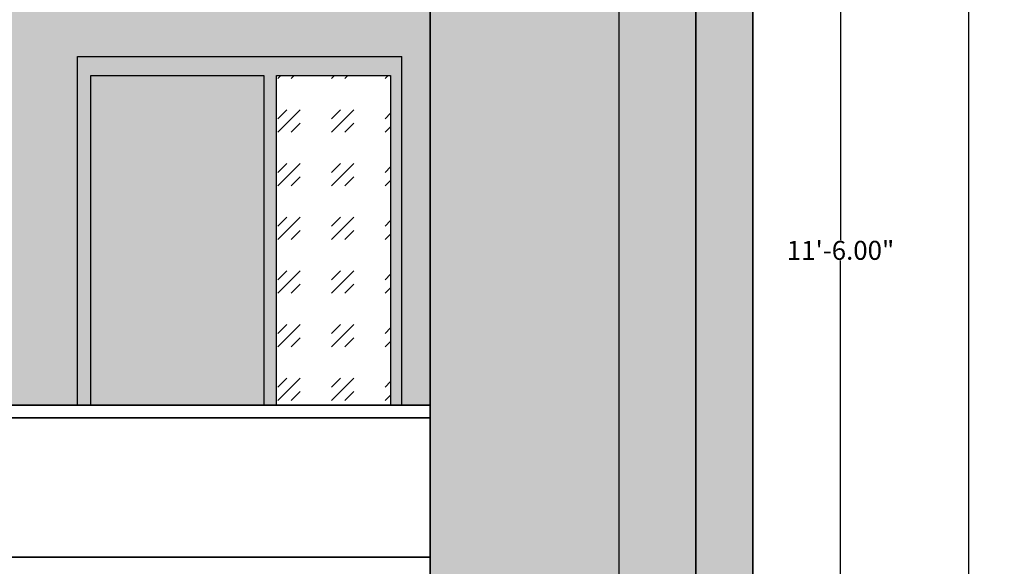
# Model space of a CAD drawing. Units: inches. Extents: x -654 to 390, y -40 to 648.
# Tile 9 of 13: x 231 to 386, y 330 to 417. Entities that reach past the tile are written whole.
import ezdxf

# ---------------------------------------------------------------- set-up
doc = ezdxf.new("R2010")
doc.units = ezdxf.units.IN
doc.header["$PDMODE"] = 3
for name, color, linetype, lineweight in [('A-ANNO-DIMS', 2, 'Continuous', 18), ('A-ELEV', 7, 'Continuous', 35), ('A-ELEV-FILL', 252, 'Continuous', 13), ('A-ELEV-PATT', 8, 'Continuous', 13), ('A-GLAZ', 4, 'Continuous', 25)]:
    doc.layers.add(name, color=color, linetype=linetype, lineweight=lineweight)
doc.styles.get("Standard").update_dxf_attribs({"font": 'arial.ttf'})
doc.dimstyles.get("Standard").update_dxf_attribs({"dimtxt": 3, "dimasz": 3, "dimexe": 0.18, "dimexo": 0.0625, "dimgap": 0.09, "dimtad": 0, "dimtih": 1, "dimtoh": 1, "dimzin": 0, "dimdsep": 46, "dimlunit": 3, "dimtxsty": 'Standard', "dimblk": 'ARCHTICK', "dimcen": 0.09, "dimse1": 1, "dimse2": 1, "dimadec": 0, "dimazin": 0, "dimtfac": 1, "dimtofl": 0, "dimtmove": 0, "dimatfit": 3, "dimfxl": 1, "dimtolj": 1, "dimtzin": 0, "dimarcsym": 0})

# ---------------------------------------------------------------- blocks, each defined once
blk = doc.blocks.new('_ArchTick')
at = {"color": 0, "linetype": 'ByBlock', "const_width": 0.15}
blk.add_lwpolyline([(-0.5, -0.5), (0.5, 0.5)], dxfattribs=at)
blk = doc.blocks.new('*D6')
at = {"layer": 'A-ANNO-DIMS', "color": 0, "lineweight": -2, "transparency": 16777216}
for p, q in [((360.51, 449.13), (360.51, 381.76)), ((360.51, 311.13), (360.51, 378.51))]:
    blk.add_line(p, q, dxfattribs=at)
at = {"layer": 'Defpoints', "color": 0, "transparency": 16777216}
for p in [(337.55, 449.13), (360.51, 449.13), (303.82, 311.13)]:
    blk.add_point(p, dxfattribs=at)
at = {"layer": 'A-ANNO-DIMS', "color": 0, "lineweight": -2, "transparency": 16777216, "xscale": 3, "yscale": 3, "zscale": 3}
for p, rotation in [((360.51, 449.13), 90), ((360.51, 311.13), 270)]:
    blk.add_blockref('_ArchTick', p, dxfattribs=dict(at, rotation=rotation))
at = {"layer": 'A-ANNO-DIMS', "color": 0, "transparency": 16777216, "insert": (360.51, 380.13), "char_height": 3, "attachment_point": 5}
blk.add_mtext('\\A1;11\'-6.00"', dxfattribs=at)
blk = doc.blocks.new('*D41')
at = {"layer": 'A-ANNO-DIMS', "color": 0, "lineweight": -2, "transparency": 16777216}
for p, q in [((325.46, 442.63), (325.46, 311.76)), ((325.46, 177.63), (325.46, 308.51))]:
    blk.add_line(p, q, dxfattribs=at)
at = {"layer": 'Defpoints', "color": 0, "transparency": 16777216}
for p in [(295.65, 442.63), (295.65, 177.63), (325.46, 177.63)]:
    blk.add_point(p, dxfattribs=at)
at = {"layer": 'A-ANNO-DIMS', "color": 0, "lineweight": -2, "transparency": 16777216, "xscale": 3, "yscale": 3, "zscale": 3}
for p, rotation in [((325.46, 442.63), 90), ((325.46, 177.63), 270)]:
    blk.add_blockref('_ArchTick', p, dxfattribs=dict(at, rotation=rotation))
at = {"layer": 'A-ANNO-DIMS', "color": 0, "transparency": 16777216, "insert": (325.46, 310.13), "char_height": 3, "attachment_point": 5}
blk.add_mtext('\\A1;22\'-1.00"', dxfattribs=at)
blk = doc.blocks.new('*D76')
at = {"layer": 'A-ANNO-DIMS', "color": 0, "lineweight": -2, "transparency": 16777216}
for p, q in [((380.75, 611.13), (380.75, 306.76)), ((380.75, -0.87), (380.75, 303.51))]:
    blk.add_line(p, q, dxfattribs=at)
at = {"layer": 'Defpoints', "color": 0, "transparency": 16777216}
for p in [(126.65, 611.13), (380.75, 611.13), (346.65, -0.87)]:
    blk.add_point(p, dxfattribs=at)
at = {"layer": 'A-ANNO-DIMS', "color": 0, "lineweight": -2, "transparency": 16777216, "xscale": 3, "yscale": 3, "zscale": 3}
for p, rotation in [((380.75, 611.13), 90), ((380.75, -0.87), 270)]:
    blk.add_blockref('_ArchTick', p, dxfattribs=dict(at, rotation=rotation))
at = {"layer": 'A-ANNO-DIMS', "color": 0, "transparency": 16777216, "insert": (380.75, 305.13), "char_height": 3, "attachment_point": 5}
blk.add_mtext('\\A1;51\'-0"', dxfattribs=at)
blk = doc.blocks.new('*D89')
at = {"layer": 'A-ANNO-DIMS', "color": 0, "lineweight": -2, "transparency": 16777216}
for p, q in [((243.65, 643.23), (287.57, 643.23)), ((339.65, 643.23), (295.73, 643.23))]:
    blk.add_line(p, q, dxfattribs=at)
at = {"layer": 'Defpoints', "color": 0, "transparency": 16777216}
for p in [(339.65, 643.23), (243.65, 17.13), (339.65, 17.13)]:
    blk.add_point(p, dxfattribs=at)
at = {"layer": 'A-ANNO-DIMS', "color": 0, "lineweight": -2, "transparency": 16777216, "xscale": 3, "yscale": 3, "zscale": 3, "rotation": 180}
blk.add_blockref('_ArchTick', (243.65, 643.23), dxfattribs=at)
at = {"layer": 'A-ANNO-DIMS', "color": 0, "lineweight": -2, "transparency": 16777216, "xscale": 3, "yscale": 3, "zscale": 3}
blk.add_blockref('_ArchTick', (339.65, 643.23), dxfattribs=at)
at = {"layer": 'A-ANNO-DIMS', "color": 0, "transparency": 16777216, "insert": (291.65, 643.23), "char_height": 3, "attachment_point": 5}
blk.add_mtext('\\A1;8\'-0"', dxfattribs=at)
blk = doc.blocks.new('*D90')
at = {"layer": 'A-ANNO-DIMS', "color": 0, "lineweight": -2, "transparency": 16777216}
for p, q in [((339.65, 643.23), (346.65, 643.23)), ((346.65, 643.23), (349.65, 643.23))]:
    blk.add_line(p, q, dxfattribs=at)
at = {"layer": 'Defpoints', "color": 0, "transparency": 16777216}
for p in [(346.65, 643.23), (339.65, 17.13), (346.65, 17.13)]:
    blk.add_point(p, dxfattribs=at)
at = {"layer": 'A-ANNO-DIMS', "color": 0, "lineweight": -2, "transparency": 16777216, "xscale": 3, "yscale": 3, "zscale": 3, "rotation": 180}
blk.add_blockref('_ArchTick', (339.65, 643.23), dxfattribs=at)
at = {"layer": 'A-ANNO-DIMS', "color": 0, "lineweight": -2, "transparency": 16777216, "xscale": 3, "yscale": 3, "zscale": 3}
blk.add_blockref('_ArchTick', (346.65, 643.23), dxfattribs=at)
at = {"layer": 'A-ANNO-DIMS', "color": 0, "transparency": 16777216, "insert": (353.72, 643.23), "char_height": 3, "attachment_point": 5}
blk.add_mtext('\\A1;0\'-7"', dxfattribs=at)
blk = doc.blocks.new('*D101')
at = {"layer": 'A-ANNO-DIMS', "color": 0, "lineweight": -2, "transparency": 16777216}
for p, q in [((-35.45, 410.79), (-35.45, 384.8)), ((-35.45, 355.63), (-35.45, 381.62))]:
    blk.add_line(p, q, dxfattribs=at)
at = {"layer": 'Defpoints', "color": 0, "transparency": 16777216}
for p in [(-35.45, 410.79), (239.87, 410.79), (239.87, 355.63)]:
    blk.add_point(p, dxfattribs=at)
at = {"layer": 'A-ANNO-DIMS', "color": 0, "lineweight": -2, "transparency": 16777216, "xscale": 3, "yscale": 3, "zscale": 3}
for p, rotation in [((-35.45, 410.79), 90), ((-35.45, 355.63), 270)]:
    blk.add_blockref('_ArchTick', p, dxfattribs=dict(at, rotation=rotation))
at = {"layer": 'A-ANNO-DIMS', "color": 0, "transparency": 16777216, "insert": (-35.45, 383.21), "char_height": 3, "attachment_point": 5}
blk.add_mtext('\\A1;4\'-7"', dxfattribs=at)
blk = doc.blocks.new('*D102')
at = {"layer": 'A-ANNO-DIMS', "color": 0, "lineweight": -2, "transparency": 16777216}
for p, q in [((179.88, -32.97), (205.8, -32.97)), ((239.87, -32.97), (213.95, -32.97))]:
    blk.add_line(p, q, dxfattribs=at)
at = {"layer": 'Defpoints', "color": 0, "transparency": 16777216}
for p in [(179.88, 355.63), (239.87, 355.63), (239.87, -32.97)]:
    blk.add_point(p, dxfattribs=at)
at = {"layer": 'A-ANNO-DIMS', "color": 0, "lineweight": -2, "transparency": 16777216, "xscale": 3, "yscale": 3, "zscale": 3, "rotation": 180}
blk.add_blockref('_ArchTick', (179.88, -32.97), dxfattribs=at)
at = {"layer": 'A-ANNO-DIMS', "color": 0, "lineweight": -2, "transparency": 16777216, "xscale": 3, "yscale": 3, "zscale": 3}
blk.add_blockref('_ArchTick', (239.87, -32.97), dxfattribs=at)
at = {"layer": 'A-ANNO-DIMS', "color": 0, "transparency": 16777216, "insert": (209.87, -32.97), "char_height": 3, "attachment_point": 5}
blk.add_mtext('\\A1;5\'-0"', dxfattribs=at)
blk = doc.blocks.new('*D103')
at = {"layer": 'A-ANNO-DIMS', "color": 0, "lineweight": -2, "transparency": 16777216}
for p, q in [((239.87, -32.97), (257.87, -32.97)), ((291.14, -32.97), (273.14, -32.97))]:
    blk.add_line(p, q, dxfattribs=at)
at = {"layer": 'Defpoints', "color": 0, "transparency": 16777216}
for p in [(239.87, 355.63), (291.14, 355.63), (291.14, -32.97)]:
    blk.add_point(p, dxfattribs=at)
at = {"layer": 'A-ANNO-DIMS', "color": 0, "lineweight": -2, "transparency": 16777216, "xscale": 3, "yscale": 3, "zscale": 3, "rotation": 180}
blk.add_blockref('_ArchTick', (239.87, -32.97), dxfattribs=at)
at = {"layer": 'A-ANNO-DIMS', "color": 0, "lineweight": -2, "transparency": 16777216, "xscale": 3, "yscale": 3, "zscale": 3}
blk.add_blockref('_ArchTick', (291.14, -32.97), dxfattribs=at)
at = {"layer": 'A-ANNO-DIMS', "color": 0, "transparency": 16777216, "insert": (265.51, -32.97), "char_height": 3, "attachment_point": 5}
blk.add_mtext('\\A1;4\'-3 1/2"', dxfattribs=at)

msp = doc.modelspace()

# ---------------------------------------------------------------- hatches: boundary and pattern name
at = {"layer": 'A-ELEV-FILL'}
h = msp.add_hatch(color=256, dxfattribs=at)
h.dxf.hatch_style = 1
h.paths.add_polyline_path([(161.035, 590.134), (-1.354, 590.134), (-1.354, 581.134), (161.035, 581.134)])
h.paths.add_polyline_path([(346.646, 453.634), (-1.354, 453.634), (-1.354, 444.634), (337.646, 444.634), (337.646, 177.634), (178.742, 177.634), (178.742, 173.134), (176.742, 173.134), (176.742, 177.634), (166.742, 177.634), (166.742, 173.134), (164.742, 173.134), (164.742, 177.634), (154.742, 177.634), (154.742, 173.134), (152.742, 173.134), (152.742, 177.634), (142.742, 177.634), (142.742, 173.134), (140.742, 173.134), (140.742, 177.634), (130.742, 177.634), (130.742, 173.134), (128.742, 173.134), (128.742, 177.634), (115.646, 177.634), (115.646, 168.634), (346.646, 168.634), (346.646, 173.134)])
h.paths.add_polyline_path([(7.646, 87.642), (-1.354, 87.642), (-1.354, 17.134), (7.646, 17.134)])
h.paths.add_polyline_path([(16.396, 116.134), (60.646, 116.134), (60.646, 83.134), (62.646, 83.134), (113.646, 83.134), (115.646, 83.134), (115.646, 125.134), (7.646, 125.134), (7.646, 89.642), (8.146, 89.642), (8.146, 87.642), (7.646, 87.642), (7.646, 83.134), (9.646, 83.134), (16.396, 83.134)])
h = msp.add_hatch(color=256, dxfattribs=at)
h.dxf.hatch_style = 1
h.paths.add_polyline_path([(41.55, 80.08), (28.05, 80.08), (28.05, 20.08), (41.55, 20.08)])
h.paths.add_polyline_path([(93.843, 80.08), (80.343, 80.08), (80.343, 20.08), (93.843, 20.08)])
h.paths.add_polyline_path([(337.646, 442.634), (295.646, 442.634), (295.646, 316.634), (304.646, 316.634), (304.646, 315.634), (303.818, 315.634), (303.818, 306.634), (304.646, 306.634), (304.646, 305.634), (295.646, 305.634), (295.646, 177.634), (337.646, 177.634)])
h.paths.add_polyline_path([(346.646, 495.134), (184.646, 495.134), (184.646, 453.634), (346.646, 453.634)])
h.paths.add_polyline_path([(198.646, 473.634), (198.646, 486.134), (332.646, 486.134), (332.646, 473.634)], flags=16)
h.paths.add_polyline_path([(199.646, 474.634), (199.646, 485.134), (331.646, 485.134), (331.646, 474.634)], flags=0)
h = msp.add_hatch(color=256, dxfattribs=at)
h.dxf.hatch_style = 1
h.paths.add_polyline_path([(239.871, 410.786), (291.141, 410.786), (291.141, 355.634), (295.646, 355.634), (295.646, 442.634), (145.646, 442.634), (145.646, 410.786), (179.877, 410.786), (179.877, 355.634), (239.871, 355.634)])
h = msp.add_hatch(color=256, dxfattribs=at)
h.dxf.hatch_style = 1
h.paths.add_polyline_path([(138.646, 438.634), (107.646, 438.634), (107.646, 359.634), (138.646, 359.634)])
h.paths.add_polyline_path([(136.646, 436.634), (136.646, 361.634), (109.646, 361.634), (109.646, 436.634)], flags=16)
h.paths.add_polyline_path([(179.877, 410.786), (145.646, 410.786), (145.646, 407.786), (153.285, 407.786), (153.285, 357.634), (145.646, 357.634), (145.646, 355.634), (179.877, 355.634)])
h.paths.add_polyline_path([(178.123, 407.786), (178.123, 357.634), (155.286, 357.634), (155.286, 407.786)], flags=16)
h.paths.add_polyline_path([(291.141, 410.786), (239.871, 410.786), (239.871, 355.634), (241.996, 355.634), (241.996, 407.786), (269.317, 407.786), (269.317, 355.634), (271.318, 355.634), (271.318, 407.786), (289.369, 407.786), (289.369, 355.634), (291.141, 355.634)])
h.paths.add_polyline_path([(128.225, 268.786), (128.742, 268.786), (128.742, 271.786), (125.225, 271.786), (125.225, 216.634), (128.225, 216.634)])
h.paths.add_polyline_path([(140.742, 271.786), (130.742, 271.786), (130.742, 268.786), (140.742, 268.786)])
h.paths.add_polyline_path([(152.742, 271.786), (142.742, 271.786), (142.742, 268.786), (152.742, 268.786)])
h.paths.add_polyline_path([(164.742, 271.786), (154.742, 271.786), (154.742, 268.786), (164.742, 268.786)])
h.paths.add_polyline_path([(176.742, 271.786), (167.328, 271.786), (166.742, 271.786), (166.742, 268.786), (167.328, 268.786), (167.328, 216.634), (169.328, 216.634), (169.328, 268.786), (176.742, 268.786)])
h.paths.add_polyline_path([(221.328, 271.786), (178.742, 271.786), (178.742, 268.786), (184.828, 268.786), (184.828, 216.634), (186.829, 216.634), (186.829, 268.786), (202.329, 268.786), (202.329, 216.634), (204.325, 216.634), (204.325, 268.786), (219.825, 268.786), (219.825, 216.634), (221.328, 216.634)])
h.paths.add_polyline_path([(295.646, 271.786), (244.726, 271.786), (244.726, 216.634), (246.481, 216.634), (246.481, 268.786), (269.317, 268.786), (269.317, 216.634), (271.318, 216.634), (271.318, 268.786), (286.818, 268.786), (286.818, 216.634), (288.814, 216.634), (288.814, 268.786), (295.646, 268.786)])
h.paths.add_polyline_path([(295.646, 216.634), (178.742, 216.634), (178.742, 214.634), (295.646, 214.634)])
h.paths.add_polyline_path([(128.742, 216.634), (123.485, 216.634), (123.485, 214.634), (128.742, 214.634)])
h.paths.add_polyline_path([(140.742, 216.634), (130.742, 216.634), (130.742, 214.634), (140.742, 214.634)])
h.paths.add_polyline_path([(152.742, 216.634), (142.742, 216.634), (142.742, 214.634), (152.742, 214.634)])
h.paths.add_polyline_path([(164.742, 216.634), (154.742, 216.634), (154.742, 214.634), (164.742, 214.634)])
h.paths.add_polyline_path([(176.742, 216.634), (166.742, 216.634), (166.742, 214.634), (176.742, 214.634)])
h.paths.add_polyline_path([(128.742, 192.634), (119.386, 192.634), (119.386, 190.634), (128.742, 190.634)])
h.paths.add_polyline_path([(140.742, 192.634), (130.742, 192.634), (130.742, 190.634), (140.742, 190.634)])
h.paths.add_polyline_path([(152.742, 192.634), (142.742, 192.634), (142.742, 190.634), (152.742, 190.634)])
h.paths.add_polyline_path([(164.742, 192.634), (154.742, 192.634), (154.742, 190.634), (164.742, 190.634)])
h.paths.add_polyline_path([(176.742, 192.634), (166.742, 192.634), (166.742, 190.634), (176.742, 190.634)])
h.paths.add_polyline_path([(295.646, 192.634), (178.742, 192.634), (178.742, 190.634), (295.646, 190.634)])
h.paths.add_polyline_path([(189.362, 137.63), (135.362, 137.63), (135.362, 71.63), (189.362, 71.63)])
h.paths.add_polyline_path([(154.862, 134.63), (170.362, 134.63), (170.362, 74.63), (154.862, 74.63)], flags=16)
h.paths.add_polyline_path([(152.862, 134.63), (152.862, 74.63), (137.362, 74.63), (137.362, 134.63)], flags=16)
h.paths.add_polyline_path([(172.358, 134.63), (187.858, 134.63), (187.858, 74.63), (172.358, 74.63)], flags=16)
h.paths.add_polyline_path([(113.646, 83.134), (62.646, 83.134), (62.646, 17.134), (113.646, 17.134)])
h.paths.add_polyline_path([(96.484, 80.08), (109.984, 80.08), (109.984, 20.08), (96.484, 20.08)], flags=16)
h.paths.add_polyline_path([(93.843, 80.08), (93.843, 20.08), (80.343, 20.08), (80.343, 80.08)], flags=16)
h.paths.add_polyline_path([(78.051, 80.08), (78.051, 20.08), (64.551, 20.08), (64.551, 80.08)], flags=16)
h.paths.add_polyline_path([(60.646, 83.134), (9.646, 83.134), (9.646, 17.134), (60.646, 17.134)])
h.paths.add_polyline_path([(58.197, 80.08), (58.197, 20.08), (44.697, 20.08), (44.697, 80.08)], flags=16)
h.paths.add_polyline_path([(41.55, 80.08), (41.55, 20.08), (28.05, 20.08), (28.05, 80.08)], flags=16)
h.paths.add_polyline_path([(25.146, 80.08), (25.146, 20.08), (11.646, 20.08), (11.646, 80.08)], flags=16)
h.paths.add_polyline_path([(9.646, 83.134), (7.646, 83.134), (7.646, 73.776), (9.646, 73.776)])
h.paths.add_polyline_path([(9.646, 65.663), (7.646, 65.663), (7.646, 36.041), (9.646, 36.041)])
h.paths.add_polyline_path([(9.646, 27.928), (7.646, 27.928), (7.646, 17.134), (9.646, 17.134)])
h.paths.add_polyline_path([(115.646, 83.134), (113.646, 83.134), (113.646, 73.776), (115.646, 73.776)])
h.paths.add_polyline_path([(115.646, 65.663), (113.646, 65.663), (113.646, 35.502), (115.646, 35.502)])
h.paths.add_polyline_path([(115.646, 27.389), (113.646, 27.389), (113.646, 17.134), (115.646, 17.134)])
h.paths.add_polyline_path([(8.146, 89.642), (-1.854, 89.642), (-1.854, 87.642), (8.146, 87.642)])
h.paths.add_polyline_path([(245.646, 156.634), (243.646, 156.634), (243.646, 17.134), (245.646, 17.134)])
h.paths.add_polyline_path([(339.646, 156.634), (337.646, 156.634), (337.646, 17.134), (339.646, 17.134)])
h = msp.add_hatch(color=256, dxfattribs=at)
h.dxf.hatch_style = 1
h.paths.add_polyline_path([(269.317, 268.786), (246.481, 268.786), (246.481, 216.634), (269.317, 216.634)])
h.paths.add_polyline_path([(269.317, 407.786), (241.996, 407.786), (241.996, 355.634), (269.317, 355.634)])
h.paths.add_polyline_path([(140.742, 268.786), (130.742, 268.786), (130.742, 216.634), (140.742, 216.634)])
h.paths.add_polyline_path([(152.742, 268.786), (142.742, 268.786), (142.742, 216.634), (152.742, 216.634)])
h.paths.add_polyline_path([(164.742, 268.786), (154.742, 268.786), (154.742, 216.634), (164.742, 216.634)])
at = {"layer": 'A-ELEV-PATT'}
h = msp.add_hatch(dxfattribs=at)
h.set_pattern_fill('GOST_GLASS', color=256)
h.paths.add_polyline_path([(289.369, 407.786), (271.318, 407.786), (271.318, 355.634), (289.369, 355.634)])
h.paths.add_polyline_path([(178.123, 407.786), (155.286, 407.786), (155.286, 357.634), (178.123, 357.634)])
h.paths.add_polyline_path([(153.285, 407.786), (145.646, 407.786), (145.646, 357.634), (153.285, 357.634)])
h.paths.add_polyline_path([(184.828, 268.786), (178.742, 268.786), (178.742, 216.634), (184.828, 216.634)])
h.paths.add_polyline_path([(176.742, 268.786), (169.328, 268.786), (169.328, 216.634), (176.742, 216.634)])
h.paths.add_polyline_path([(202.329, 268.786), (186.829, 268.786), (186.829, 216.634), (202.329, 216.634)])
h.paths.add_polyline_path([(219.825, 268.786), (204.325, 268.786), (204.325, 216.634), (219.825, 216.634)])
h.paths.add_polyline_path([(286.818, 268.786), (271.318, 268.786), (271.318, 216.634), (286.818, 216.634)])
h.paths.add_polyline_path([(295.646, 268.786), (288.814, 268.786), (288.814, 216.634), (295.646, 216.634)])

# ---------------------------------------------------------------- linework, layer by layer
at = {"layer": 'A-ELEV'}
for p, q in [((346.646, -0.866), (346.646, 587.634)), ((337.646, 444.634), (337.646, 177.634)), ((295.646, 442.634), (295.646, 177.634)), ((145.646, 355.634), (295.646, 355.634)), ((145.646, 353.634), (295.646, 353.634)), ((145.646, 331.634), (295.646, 331.634))]:
    msp.add_line(p, q, dxfattribs=at)
at = {"layer": 'A-GLAZ'}
for points in [[(239.871, 355.634), (239.871, 410.786), (291.141, 410.786)], [(291.141, 355.634), (291.141, 410.786)], [(241.996, 355.634), (241.996, 407.786), (269.317, 407.786), (269.317, 355.634)], [(271.318, 355.634), (271.318, 407.786), (289.369, 407.786), (289.369, 355.634)]]:
    msp.add_lwpolyline(points, dxfattribs=at)

# ---------------------------------------------------------------- dimensions: what is measured, and where the dimension line sits
at = {"layer": 'A-ANNO-DIMS'}
for base, p1, p2, picture, middle in [((339.646, 643.234), (243.646, 17.134), (339.646, 17.134), '*D89', (291.646, 643.234)), ((346.646, 643.234), (339.646, 17.134), (346.646, 17.134), '*D90', (353.724, 643.234)), ((239.871, -32.966), (179.877, 355.634), (239.871, 355.634), '*D102', (209.874, -32.966)), ((291.141, -32.966), (239.871, 355.634), (291.141, 355.634), '*D103', (265.506, -32.966))]:
    dim = msp.add_linear_dim(base=base, p1=p1, p2=p2, dimstyle='Standard', override={"dimdec": 1, "dimlfac": 1, "dimrnd": 0, "dimzin": 1, "dimdsep": 46, "dimlunit": 4, "dimfrac": 2}, dxfattribs=at)
    dim.commit()
    dim.dimension.update_dxf_attribs({"geometry": picture, "text_midpoint": middle})
for base, p1, p2, override, picture, middle in [((380.746, 611.134), (346.646, -0.866), (126.646, 611.134), {"dimdec": 1, "dimlfac": 1, "dimrnd": 0, "dimzin": 1, "dimdsep": 46, "dimlunit": 4, "dimfrac": 2}, '*D76', (380.746, 305.134)), ((360.508, 449.134), (303.818, 311.134), (337.554, 449.134), {"dimclrd": 0, "dimclre": 0, "dimclrt": 0, "dimtmove": 1}, '*D6', (360.508, 380.134)), ((325.461, 177.634), (295.646, 442.634), (295.646, 177.634), {"dimclrd": 0, "dimclre": 0, "dimclrt": 0}, '*D41', (325.461, 310.134)), ((-35.454, 410.786), (239.871, 355.634), (239.871, 410.786), {"dimdec": 1, "dimlfac": 1, "dimrnd": 0, "dimzin": 1, "dimdsep": 46, "dimlunit": 4, "dimfrac": 2}, '*D101', (-35.454, 383.21))]:
    dim = msp.add_linear_dim(base=base, p1=p1, p2=p2, angle=90, dimstyle='Standard', override=override, dxfattribs=at)
    dim.commit()
    dim.dimension.update_dxf_attribs({"geometry": picture, "text_midpoint": middle})

doc.saveas('drawing.dxf')
